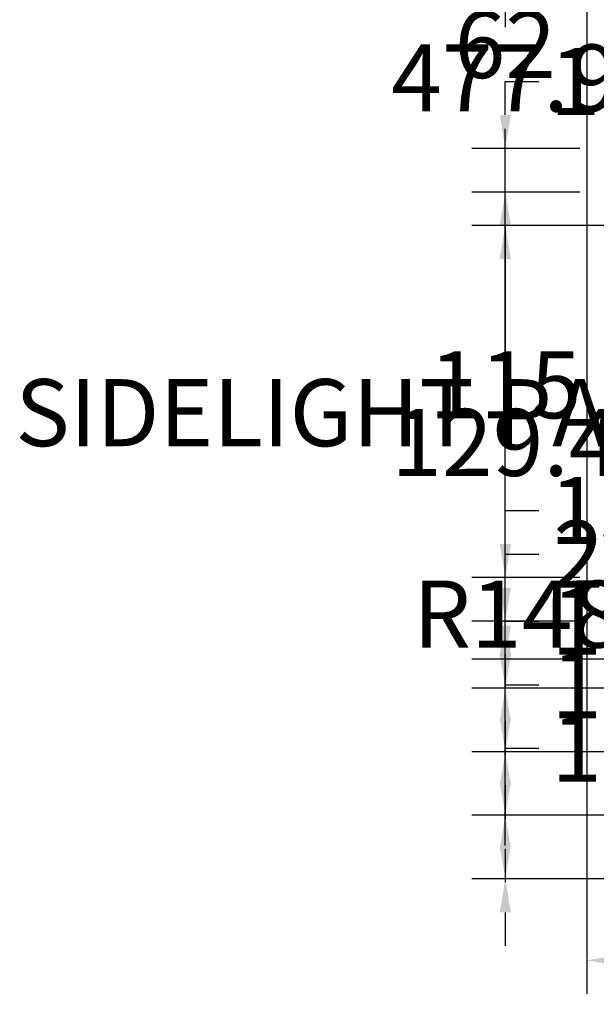
# Model space of a CAD drawing. Units: millimetres. Extents: x 130 to 1021, y 147 to 699.
# Tile 1 of 40: x 130 to 302, y 147 to 440. Entities that reach past the tile are written whole.
import ezdxf

# ---------------------------------------------------------------- set-up
doc = ezdxf.new("R2010")
doc.units = ezdxf.units.MM
doc.header["$MEASUREMENT"] = 0
doc.layers.add('A-ANNO-DIMS', color=2, linetype='Continuous', lineweight=18)
doc.styles.get("Standard").update_dxf_attribs({"font": 'arial.ttf'})
doc.dimstyles.get("Standard").update_dxf_attribs({"dimtxt": 20, "dimasz": 10, "dimexe": 10, "dimexo": 10, "dimgap": 5, "dimtad": 0, "dimtih": 1, "dimtoh": 1, "dimdec": 0, "dimzin": 0, "dimdsep": 46, "dimtxsty": 'Standard', "dimcen": 5, "dimadec": 0, "dimazin": 0, "dimtfac": 1, "dimtdec": 0, "dimtofl": 0, "dimtmove": 0, "dimatfit": 3, "dimfxl": 1, "dimtolj": 1, "dimtzin": 0, "dimarcsym": 0})

# ---------------------------------------------------------------- blocks, each defined once
blk = doc.blocks.new('*D9')
at = {"layer": 'A-ANNO-DIMS', "color": 0, "lineweight": -2, "transparency": 16777216}
for p, q in [((467.37, 323.13), (457.37, 323.13)), ((467.37, 313.13), (467.37, 323.13)), ((473.55, 303.13), (477.38, 303.13)), ((473.57, 277.58), (477.4, 277.58)), ((467.41, 267.57), (467.42, 257.57))]:
    blk.add_line(p, q, dxfattribs=at)
at = {"layer": 'A-ANNO-DIMS', "color": 0, "transparency": 16777216}
for points in [[(469.04, 313.13), (465.71, 313.13), (467.38, 303.13)], [(469.08, 267.57), (465.75, 267.57), (467.4, 277.57)]]:
    blk.add_solid(points, dxfattribs=at)
at = {"layer": 'Defpoints', "color": 0, "transparency": 16777216}
for p in [(463.55, 303.12), (467.38, 303.13), (463.57, 277.57)]:
    blk.add_point(p, dxfattribs=at)
at = {"layer": 'A-ANNO-DIMS', "color": 0, "transparency": 16777216, "insert": (284.19, 323.13), "char_height": 20, "attachment_point": 5}
blk.add_mtext('\\A1;SIDELIGHT PANE 26 TYP.', dxfattribs=at)
blk = doc.blocks.new('*D11')
at = {"layer": 'A-ANNO-DIMS', "color": 0, "lineweight": -2, "transparency": 16777216}
for p, q in [((737.37, 648.7), (737.37, 149.74)), ((299.37, 566.95), (299.37, 149.74)), ((309.37, 159.74), (490.86, 159.74)), ((727.37, 159.74), (545.89, 159.74))]:
    blk.add_line(p, q, dxfattribs=at)
at = {"layer": 'A-ANNO-DIMS', "color": 0, "transparency": 16777216}
for points in [[(309.37, 161.41), (309.37, 158.07), (299.37, 159.74)], [(727.37, 161.41), (727.37, 158.07), (737.37, 159.74)]]:
    blk.add_solid(points, dxfattribs=at)
at = {"layer": 'Defpoints', "color": 0, "transparency": 16777216}
for p in [(737.37, 658.7), (299.37, 576.95), (737.37, 159.74)]:
    blk.add_point(p, dxfattribs=at)
at = {"layer": 'A-ANNO-DIMS', "color": 0, "transparency": 16777216, "insert": (518.37, 159.74), "char_height": 20, "attachment_point": 5}
blk.add_mtext('\\A1;438', dxfattribs=at)
blk = doc.blocks.new('*D12')
at = {"layer": 'A-ANNO-DIMS', "color": 0, "lineweight": -2, "transparency": 16777216}
for p, q in [((477.37, 661.95), (265.07, 661.95)), ((275.07, 651.95), (275.07, 438.2)), ((275.07, 194.04), (275.07, 407.78)), ((357.16, 184.04), (265.07, 184.04))]:
    blk.add_line(p, q, dxfattribs=at)
at = {"layer": 'A-ANNO-DIMS', "color": 0, "transparency": 16777216}
for points in [[(273.41, 651.95), (276.74, 651.95), (275.07, 661.95)], [(273.41, 194.04), (276.74, 194.04), (275.07, 184.04)]]:
    blk.add_solid(points, dxfattribs=at)
at = {"layer": 'Defpoints', "color": 0, "transparency": 16777216}
for p in [(275.07, 661.95), (487.37, 661.95), (367.16, 184.04)]:
    blk.add_point(p, dxfattribs=at)
at = {"layer": 'A-ANNO-DIMS', "color": 0, "transparency": 16777216, "insert": (275.07, 422.99), "char_height": 20, "attachment_point": 5}
blk.add_mtext('\\A1;477.9', dxfattribs=at)
blk = doc.blocks.new('*D33')
at = {"layer": 'A-ANNO-DIMS', "color": 0, "lineweight": -2, "transparency": 16777216}
for p, q in [((275.07, 213.01), (275.07, 223.01)), ((275.07, 223.01), (285.07, 223.01)), ((462.91, 203.01), (265.07, 203.01)), ((357.16, 184.04), (265.07, 184.04)), ((275.07, 174.04), (275.07, 164.04))]:
    blk.add_line(p, q, dxfattribs=at)
at = {"layer": 'A-ANNO-DIMS', "color": 0, "transparency": 16777216}
for points in [[(273.41, 213.01), (276.74, 213.01), (275.07, 203.01)], [(273.41, 174.04), (276.74, 174.04), (275.07, 184.04)]]:
    blk.add_solid(points, dxfattribs=at)
at = {"layer": 'Defpoints', "color": 0, "transparency": 16777216}
for p in [(275.07, 203.01), (472.91, 203.01), (367.16, 184.04)]:
    blk.add_point(p, dxfattribs=at)
at = {"layer": 'A-ANNO-DIMS', "color": 0, "transparency": 16777216, "insert": (322.88, 223.01), "char_height": 20, "attachment_point": 5}
blk.add_mtext('\\A1;18.97', dxfattribs=at)
blk = doc.blocks.new('*D34')
at = {"layer": 'A-ANNO-DIMS', "color": 0, "lineweight": -2, "transparency": 16777216}
for p, q in [((275.07, 231.98), (275.07, 241.98)), ((275.07, 241.98), (285.07, 241.98)), ((459.84, 221.98), (265.07, 221.98)), ((462.91, 203.01), (265.07, 203.01)), ((275.07, 193.01), (275.07, 183.01))]:
    blk.add_line(p, q, dxfattribs=at)
at = {"layer": 'A-ANNO-DIMS', "color": 0, "transparency": 16777216}
for points in [[(273.41, 231.98), (276.74, 231.98), (275.07, 221.98)], [(273.41, 193.01), (276.74, 193.01), (275.07, 203.01)]]:
    blk.add_solid(points, dxfattribs=at)
at = {"layer": 'Defpoints', "color": 0, "transparency": 16777216}
for p in [(275.07, 221.98), (469.84, 221.98), (472.91, 203.01)]:
    blk.add_point(p, dxfattribs=at)
at = {"layer": 'A-ANNO-DIMS', "color": 0, "transparency": 16777216, "insert": (322.88, 241.98), "char_height": 20, "attachment_point": 5}
blk.add_mtext('\\A1;18.97', dxfattribs=at)
blk = doc.blocks.new('*D35')
at = {"layer": 'A-ANNO-DIMS', "color": 0, "lineweight": -2, "transparency": 16777216}
for p, q in [((275.07, 250.95), (275.07, 260.95)), ((275.07, 260.95), (285.07, 260.95)), ((456.77, 240.95), (265.07, 240.95)), ((459.84, 221.98), (265.07, 221.98)), ((275.07, 211.98), (275.07, 201.98))]:
    blk.add_line(p, q, dxfattribs=at)
at = {"layer": 'A-ANNO-DIMS', "color": 0, "transparency": 16777216}
for points in [[(273.41, 250.95), (276.74, 250.95), (275.07, 240.95)], [(273.41, 211.98), (276.74, 211.98), (275.07, 221.98)]]:
    blk.add_solid(points, dxfattribs=at)
at = {"layer": 'Defpoints', "color": 0, "transparency": 16777216}
for p in [(275.07, 240.95), (466.77, 240.95), (469.84, 221.98)]:
    blk.add_point(p, dxfattribs=at)
at = {"layer": 'A-ANNO-DIMS', "color": 0, "transparency": 16777216, "insert": (322.88, 260.95), "char_height": 20, "attachment_point": 5}
blk.add_mtext('\\A1;18.97', dxfattribs=at)
blk = doc.blocks.new('*D36')
at = {"layer": 'A-ANNO-DIMS', "color": 0, "lineweight": -2, "transparency": 16777216}
for p, q in [((275.07, 270.95), (275.07, 280.95)), ((275.07, 280.95), (285.07, 280.95)), ((297.37, 260.95), (265.07, 260.95)), ((456.77, 240.95), (265.07, 240.95)), ((275.07, 230.95), (275.07, 220.95))]:
    blk.add_line(p, q, dxfattribs=at)
at = {"layer": 'A-ANNO-DIMS', "color": 0, "transparency": 16777216}
for points in [[(273.41, 270.95), (276.74, 270.95), (275.07, 260.95)], [(273.41, 230.95), (276.74, 230.95), (275.07, 240.95)]]:
    blk.add_solid(points, dxfattribs=at)
at = {"layer": 'Defpoints', "color": 0, "transparency": 16777216}
for p in [(275.07, 260.95), (307.37, 260.95), (466.77, 240.95)]:
    blk.add_point(p, dxfattribs=at)
at = {"layer": 'A-ANNO-DIMS', "color": 0, "transparency": 16777216, "insert": (304.53, 280.95), "char_height": 20, "attachment_point": 5}
blk.add_mtext('\\A1;20', dxfattribs=at)
blk = doc.blocks.new('*D37')
at = {"layer": 'A-ANNO-DIMS', "color": 0, "lineweight": -2, "transparency": 16777216}
for p, q in [((275.07, 283.95), (275.07, 293.95)), ((275.07, 293.95), (285.07, 293.95)), ((297.37, 273.95), (265.07, 273.95)), ((297.37, 260.95), (265.07, 260.95)), ((275.07, 250.95), (275.07, 240.95))]:
    blk.add_line(p, q, dxfattribs=at)
at = {"layer": 'A-ANNO-DIMS', "color": 0, "transparency": 16777216}
for points in [[(273.41, 283.95), (276.74, 283.95), (275.07, 273.95)], [(273.41, 250.95), (276.74, 250.95), (275.07, 260.95)]]:
    blk.add_solid(points, dxfattribs=at)
at = {"layer": 'Defpoints', "color": 0, "transparency": 16777216}
for p in [(275.07, 273.95), (307.37, 273.95), (307.37, 260.95)]:
    blk.add_point(p, dxfattribs=at)
at = {"layer": 'A-ANNO-DIMS', "color": 0, "transparency": 16777216, "insert": (303.46, 293.95), "char_height": 20, "attachment_point": 5}
blk.add_mtext('\\A1;13', dxfattribs=at)
blk = doc.blocks.new('*D38')
at = {"layer": 'A-ANNO-DIMS', "color": 0, "lineweight": -2, "transparency": 16777216}
for p, q in [((297.37, 388.95), (265.07, 388.95)), ((275.07, 378.95), (275.07, 346.66)), ((275.07, 283.95), (275.07, 316.24)), ((297.37, 273.95), (265.07, 273.95))]:
    blk.add_line(p, q, dxfattribs=at)
at = {"layer": 'A-ANNO-DIMS', "color": 0, "transparency": 16777216}
for points in [[(273.41, 378.95), (276.74, 378.95), (275.07, 388.95)], [(273.41, 283.95), (276.74, 283.95), (275.07, 273.95)]]:
    blk.add_solid(points, dxfattribs=at)
at = {"layer": 'Defpoints', "color": 0, "transparency": 16777216}
for p in [(275.07, 388.95), (307.37, 388.95), (307.37, 273.95)]:
    blk.add_point(p, dxfattribs=at)
at = {"layer": 'A-ANNO-DIMS', "color": 0, "transparency": 16777216, "insert": (275.07, 331.45), "char_height": 20, "attachment_point": 5}
blk.add_mtext('\\A1;115', dxfattribs=at)
blk = doc.blocks.new('*D39')
at = {"layer": 'A-ANNO-DIMS', "color": 0, "lineweight": -2, "transparency": 16777216}
for p, q in [((275.07, 411.95), (275.07, 421.95)), ((275.07, 421.95), (285.07, 421.95)), ((297.37, 401.95), (265.07, 401.95)), ((297.37, 388.95), (265.07, 388.95)), ((275.07, 378.95), (275.07, 368.95))]:
    blk.add_line(p, q, dxfattribs=at)
at = {"layer": 'A-ANNO-DIMS', "color": 0, "transparency": 16777216}
for points in [[(273.41, 411.95), (276.74, 411.95), (275.07, 401.95)], [(273.41, 378.95), (276.74, 378.95), (275.07, 388.95)]]:
    blk.add_solid(points, dxfattribs=at)
at = {"layer": 'Defpoints', "color": 0, "transparency": 16777216}
for p in [(275.07, 401.95), (307.37, 401.95), (307.37, 388.95)]:
    blk.add_point(p, dxfattribs=at)
at = {"layer": 'A-ANNO-DIMS', "color": 0, "transparency": 16777216, "insert": (303.46, 421.95), "char_height": 20, "attachment_point": 5}
blk.add_mtext('\\A1;13', dxfattribs=at)
blk = doc.blocks.new('*D40')
at = {"layer": 'A-ANNO-DIMS', "color": 0, "lineweight": -2, "transparency": 16777216}
for p, q in [((292.37, 463.95), (265.07, 463.95)), ((275.07, 453.95), (275.07, 448.16)), ((275.07, 411.95), (275.07, 417.74)), ((297.37, 401.95), (265.07, 401.95))]:
    blk.add_line(p, q, dxfattribs=at)
at = {"layer": 'A-ANNO-DIMS', "color": 0, "transparency": 16777216}
for points in [[(273.41, 453.95), (276.74, 453.95), (275.07, 463.95)], [(273.41, 411.95), (276.74, 411.95), (275.07, 401.95)]]:
    blk.add_solid(points, dxfattribs=at)
at = {"layer": 'Defpoints', "color": 0, "transparency": 16777216}
for p in [(275.07, 463.95), (302.37, 463.95), (307.37, 401.95)]:
    blk.add_point(p, dxfattribs=at)
at = {"layer": 'A-ANNO-DIMS', "color": 0, "transparency": 16777216, "insert": (275.07, 432.95), "char_height": 20, "attachment_point": 5}
blk.add_mtext('\\A1;62', dxfattribs=at)
blk = doc.blocks.new('*D60')
at = {"layer": 'A-ANNO-DIMS', "color": 0, "lineweight": -2, "transparency": 16777216}
for p, q in [((372.37, 378.95), (265.07, 378.95)), ((275.07, 368.95), (275.07, 329.46)), ((275.07, 259.55), (275.07, 299.04)), ((372.37, 249.55), (265.07, 249.55))]:
    blk.add_line(p, q, dxfattribs=at)
at = {"layer": 'A-ANNO-DIMS', "color": 0, "transparency": 16777216}
for points in [[(273.41, 368.95), (276.74, 368.95), (275.07, 378.95)], [(273.41, 259.55), (276.74, 259.55), (275.07, 249.55)]]:
    blk.add_solid(points, dxfattribs=at)
at = {"layer": 'Defpoints', "color": 0, "transparency": 16777216}
for p in [(275.07, 378.95), (382.37, 378.95), (382.37, 249.55)]:
    blk.add_point(p, dxfattribs=at)
at = {"layer": 'A-ANNO-DIMS', "color": 0, "transparency": 16777216, "insert": (275.07, 314.25), "char_height": 20, "attachment_point": 5}
blk.add_mtext('\\A1;129.4', dxfattribs=at)
blk = doc.blocks.new('*D64')
at = {"layer": 'A-ANNO-DIMS', "color": 0, "lineweight": -2, "transparency": 16777216}
for p, q in [((502.05, 450.93), (502.05, 460.93)), ((497.05, 455.93), (507.05, 455.93)), ((363.96, 263.06), (409.92, 327.25)), ((353.96, 263.06), (363.96, 263.06))]:
    blk.add_line(p, q, dxfattribs=at)
at = {"layer": 'A-ANNO-DIMS', "color": 0, "transparency": 16777216}
blk.add_solid([(408.57, 328.22), (411.28, 326.28), (415.74, 335.39)], dxfattribs=at)
at = {"layer": 'Defpoints', "color": 0, "transparency": 16777216}
for p in [(502.05, 455.93), (415.74, 335.39)]:
    blk.add_point(p, dxfattribs=at)
at = {"layer": 'A-ANNO-DIMS', "color": 0, "transparency": 16777216, "insert": (297.8, 263.06), "char_height": 20, "attachment_point": 5}
blk.add_mtext('\\A1;R148.25', dxfattribs=at)
blk = doc.blocks.new('*D66')
at = {"layer": 'A-ANNO-DIMS', "color": 0, "lineweight": -2, "transparency": 16777216}
for p, q in [((341.58, 557.19), (351.58, 557.19)), ((351.58, 557.19), (376.95, 478.14)), ((427.37, 315.98), (427.37, 325.98)), ((422.37, 320.98), (432.37, 320.98))]:
    blk.add_line(p, q, dxfattribs=at)
at = {"layer": 'A-ANNO-DIMS', "color": 0, "transparency": 16777216}
blk.add_solid([(378.53, 478.64), (375.36, 477.63), (380, 468.61)], dxfattribs=at)
at = {"layer": 'Defpoints', "color": 0, "transparency": 16777216}
for p in [(380, 468.61), (427.37, 320.98)]:
    blk.add_point(p, dxfattribs=at)
at = {"layer": 'A-ANNO-DIMS', "color": 0, "transparency": 16777216, "insert": (263.53, 557.19), "char_height": 20, "attachment_point": 5}
blk.add_mtext('\\A1;4X R155.05', dxfattribs=at)
blk = doc.blocks.new('*D68')
at = {"layer": 'A-ANNO-DIMS', "color": 0, "lineweight": -2, "transparency": 16777216}
for p, q in [((361.84, 579.76), (371.84, 579.76)), ((371.84, 579.76), (392.17, 506.69)), ((433.19, 354.23), (433.19, 364.23)), ((428.19, 359.23), (438.19, 359.23))]:
    blk.add_line(p, q, dxfattribs=at)
at = {"layer": 'A-ANNO-DIMS', "color": 0, "transparency": 16777216}
blk.add_solid([(393.77, 507.14), (390.56, 506.25), (394.85, 497.06)], dxfattribs=at)
at = {"layer": 'Defpoints', "color": 0, "transparency": 16777216}
for p in [(394.85, 497.06), (433.19, 359.23)]:
    blk.add_point(p, dxfattribs=at)
at = {"layer": 'A-ANNO-DIMS', "color": 0, "transparency": 16777216, "insert": (305.76, 579.76), "char_height": 20, "attachment_point": 5}
blk.add_mtext('\\A1;R143.06', dxfattribs=at)
blk = doc.blocks.new('*D70')
at = {"layer": 'A-ANNO-DIMS', "color": 0, "lineweight": -2, "transparency": 16777216}
for p, q in [((370.14, 588.4), (380.14, 588.4)), ((380.14, 588.4), (397.47, 517.01)), ((432.65, 367.11), (432.65, 377.11)), ((427.65, 372.11), (437.65, 372.11))]:
    blk.add_line(p, q, dxfattribs=at)
at = {"layer": 'A-ANNO-DIMS', "color": 0, "transparency": 16777216}
blk.add_solid([(399.09, 517.4), (395.85, 516.62), (399.83, 507.29)], dxfattribs=at)
at = {"layer": 'Defpoints', "color": 0, "transparency": 16777216}
for p in [(399.83, 507.29), (432.65, 372.11)]:
    blk.add_point(p, dxfattribs=at)
at = {"layer": 'A-ANNO-DIMS', "color": 0, "transparency": 16777216, "insert": (323.76, 588.4), "char_height": 20, "attachment_point": 5}
blk.add_mtext('\\A1;R139.1', dxfattribs=at)
blk = doc.blocks.new('*D73')
at = {"layer": 'A-ANNO-DIMS', "color": 0, "lineweight": -2, "transparency": 16777216}
for p, q in [((402.68, 571.45), (412.68, 571.45)), ((412.68, 571.45), (419.05, 502.17)), ((432.11, 355.14), (432.11, 365.14)), ((427.11, 360.14), (437.11, 360.14))]:
    blk.add_line(p, q, dxfattribs=at)
at = {"layer": 'A-ANNO-DIMS', "color": 0, "transparency": 16777216}
blk.add_solid([(420.71, 502.32), (417.39, 502.01), (419.97, 492.21)], dxfattribs=at)
at = {"layer": 'Defpoints', "color": 0, "transparency": 16777216}
for p in [(419.97, 492.21), (432.11, 360.14)]:
    blk.add_point(p, dxfattribs=at)
at = {"layer": 'A-ANNO-DIMS', "color": 0, "transparency": 16777216, "insert": (346.7, 571.45), "char_height": 20, "attachment_point": 5}
blk.add_mtext('\\A1;R132.62', dxfattribs=at)

msp = doc.modelspace()

# ---------------------------------------------------------------- dimensions: what is measured, and where the dimension line sits
at = {"layer": 'A-ANNO-DIMS'}
for base, p1, p2, override, picture, middle in [((275.0738, 661.9473), (367.163, 184.0395), (487.3738, 661.9473), {"dimdec": 1, "dimlfac": 1, "dimrnd": 0, "dimzin": 0, "dimdsep": 46, "dimlunit": 2}, '*D12', (275.0738, 422.9934)), ((275.0738, 463.9473), (307.3738, 401.9473), (302.3738, 463.9473), {"dimdec": 0, "dimlfac": 1, "dimrnd": 0, "dimzin": 0, "dimdsep": 46, "dimlunit": 2}, '*D40', (275.0738, 432.9473)), ((275.0738, 401.9473), (307.3738, 388.9473), (307.3738, 401.9473), {"dimdec": 0, "dimlfac": 1, "dimrnd": 0, "dimzin": 0, "dimdsep": 46, "dimlunit": 2}, '*D39', (303.4571, 421.9473)), ((275.0738, 388.9473), (307.3738, 273.9473), (307.3738, 388.9473), {"dimdec": 0, "dimlfac": 1, "dimrnd": 0, "dimzin": 0, "dimdsep": 46, "dimlunit": 2}, '*D38', (275.0738, 331.4473)), ((275.0738, 378.9473), (382.3738, 249.5473), (382.3738, 378.9473), {"dimdec": 1, "dimlfac": 1, "dimrnd": 0, "dimzin": 0, "dimdsep": 46, "dimlunit": 2}, '*D60', (275.0738, 314.2473)), ((275.0738, 273.9473), (307.3738, 260.9473), (307.3738, 273.9473), {"dimdec": 0, "dimlfac": 1, "dimrnd": 0, "dimzin": 0, "dimdsep": 46, "dimlunit": 2}, '*D37', (303.4571, 293.9473)), ((275.0738, 260.9473), (466.7667, 240.9473), (307.3738, 260.9473), {"dimdec": 0, "dimlfac": 1, "dimrnd": 0, "dimzin": 0, "dimdsep": 46, "dimlunit": 2}, '*D36', (304.5349, 280.9473)), ((275.0738, 240.9473), (469.8406, 221.978), (466.7667, 240.9473), {"dimdec": 2, "dimlfac": 1, "dimrnd": 0, "dimzin": 0, "dimdsep": 46, "dimlunit": 2}, '*D35', (322.8773, 260.9473)), ((275.0738, 221.978), (472.9145, 203.0087), (469.8406, 221.978), {"dimdec": 2, "dimlfac": 1, "dimrnd": 0, "dimzin": 0, "dimdsep": 46, "dimlunit": 2}, '*D34', (322.8773, 241.978)), ((275.0738, 203.0087), (367.163, 184.0395), (472.9145, 203.0087), {"dimdec": 2, "dimlfac": 1, "dimrnd": 0, "dimzin": 0, "dimdsep": 46, "dimlunit": 2}, '*D33', (322.8773, 223.0087))]:
    dim = msp.add_linear_dim(base=base, p1=p1, p2=p2, angle=90, dimstyle='Standard', override=override, dxfattribs=at)
    dim.commit()
    dim.dimension.update_dxf_attribs({"geometry": picture, "text_midpoint": middle})
dim = msp.add_linear_dim(base=(737.3738, 159.7395), p1=(299.3738, 576.9473), p2=(737.3738, 658.6988), dimstyle='Standard', override={"dimdec": 0, "dimlfac": 1, "dimrnd": 0, "dimzin": 0, "dimdsep": 46, "dimlunit": 2}, dxfattribs=at)
dim.commit()
dim.dimension.update_dxf_attribs({"geometry": '*D11', "text_midpoint": (518.3738, 159.7395)})
for center, mpoint, override, picture, middle in [((432.6505, 372.1087), (399.8323, 507.2907), {"dimdec": 1, "dimlfac": 1, "dimrnd": 0, "dimzin": 0, "dimdsep": 46, "dimlunit": 2}, '*D70', (323.7567, 588.3999)), ((433.1906, 359.2304), (394.8473, 497.0587), {"dimdec": 2, "dimlfac": 1, "dimrnd": 0, "dimzin": 0, "dimdsep": 46, "dimlunit": 2}, '*D68', (305.7636, 579.7557)), ((432.115, 360.1423), (419.967, 492.2083), {"dimdec": 2, "dimlfac": 1, "dimrnd": 0, "dimzin": 0, "dimdsep": 46, "dimlunit": 2}, '*D73', (346.696, 571.4479)), ((502.0489, 455.9263), (415.7433, 335.3854), {"dimdec": 2, "dimlfac": 1, "dimrnd": 0, "dimzin": 0, "dimdsep": 46, "dimlunit": 2}, '*D64', (297.8003, 263.0608))]:
    dim = msp.add_radius_dim(center=center, mpoint=mpoint, dimstyle='Standard', override=override, dxfattribs=at)
    dim.commit()
    dim.dimension.update_dxf_attribs({"geometry": picture, "text_midpoint": middle, "dimtype": 164})
dim = msp.add_radius_dim(center=(427.3738, 320.9781), mpoint=(380.0022, 468.6132), text='4X <>', dimstyle='Standard', override={"dimdec": 2, "dimlfac": 1, "dimrnd": 0, "dimzin": 0, "dimdsep": 46, "dimlunit": 2}, dxfattribs=at)
dim.commit()
dim.dimension.update_dxf_attribs({"geometry": '*D66', "text_midpoint": (263.5301, 557.1943), "dimtype": 164})
dim = msp.add_linear_dim(base=(467.3831, 303.1266), p1=(463.5714, 277.5701), p2=(463.5501, 303.1234), angle=90.047753, text='SIDELIGHT PANE <> TYP.', dimstyle='Standard', override={"dimdec": 0, "dimrnd": 0, "dimzin": 0, "dimlunit": 2}, dxfattribs=at)
dim.commit()
dim.dimension.update_dxf_attribs({"geometry": '*D9', "text_midpoint": (284.1877, 323.1266)})

doc.saveas('drawing.dxf')
